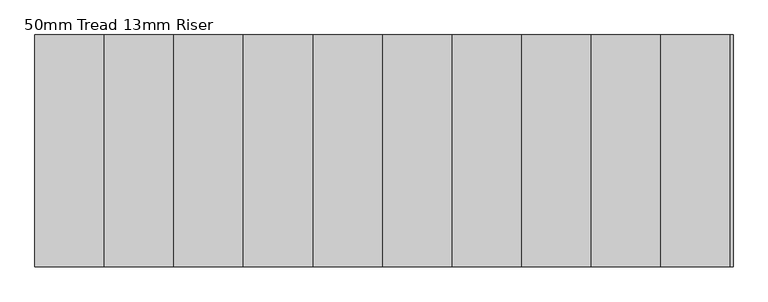
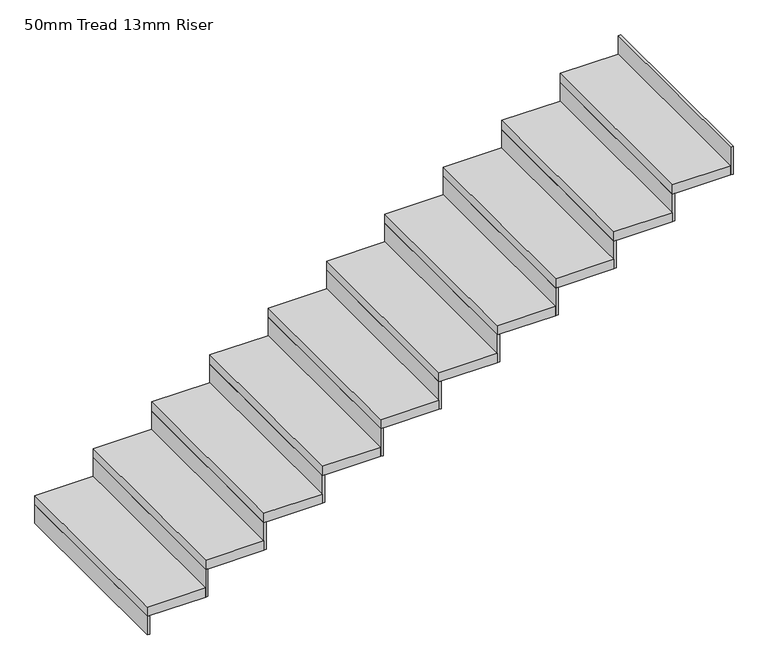
"""IFC4 building model written with IfcOpenShell, lengths in millimetres: stair flight geometry, 50mm Tread 13mm Riser."""

from ifc_helpers import new_model, si_unit, frame, origin, origin_with_axes, place, context, project, spatial, polyline, outline, extrude, source, transform, mapped, element, save


def stair_flight_50mm_tread_13mm_riser_b7d47cc6(model_context):
    return source(origin(), model_context, "Body", "SweptSolid", [
        extrude(outline(polyline([(1701.3435815, -3974.091395), (1688.8435815, -3974.091395), (1688.8435815, -2974.091395), (1701.3435815, -2974.091395), (1701.3435815, -3974.091395)])), origin_with_axes(), (0.0, 0.0, 1.0), 100.0),
        extrude(outline(polyline([(1988.8435815, -2974.091395), (1988.8435815, -3974.091395), (1688.8435815, -3974.091395), (1688.8435815, -2974.091395), (1988.8435815, -2974.091395)])), frame((0.0, 0.0, 100.0), z_axis=(0.0, 0.0, 1.0), x_axis=(1.0, 0.0, 0.0)), (0.0, 0.0, 1.0), 50.0),
        extrude(outline(polyline([(2001.3435815, -3974.091395), (1988.8435815, -3974.091395), (1988.8435815, -2974.091395), (2001.3435815, -2974.091395), (2001.3435815, -3974.091395)])), frame((0.0, 0.0, 100.0), z_axis=(0.0, 0.0, 1.0), x_axis=(1.0, 0.0, 0.0)), (0.0, 0.0, 1.0), 150.0),
        extrude(outline(polyline([(2288.8435815, -2974.091395), (2288.8435815, -3974.091395), (1988.8435815, -3974.091395), (1988.8435815, -2974.091395), (2288.8435815, -2974.091395)])), frame((0.0, 0.0, 250.0), z_axis=(0.0, 0.0, 1.0), x_axis=(1.0, 0.0, 0.0)), (0.0, 0.0, 1.0), 50.0),
        extrude(outline(polyline([(2301.3435815, -3974.091395), (2288.8435815, -3974.091395), (2288.8435815, -2974.091395), (2301.3435815, -2974.091395), (2301.3435815, -3974.091395)])), frame((0.0, 0.0, 250.0), z_axis=(0.0, 0.0, 1.0), x_axis=(1.0, 0.0, 0.0)), (0.0, 0.0, 1.0), 150.0),
        extrude(outline(polyline([(2588.8435815, -2974.091395), (2588.8435815, -3974.091395), (2288.8435815, -3974.091395), (2288.8435815, -2974.091395), (2588.8435815, -2974.091395)])), frame((0.0, 0.0, 400.0), z_axis=(0.0, 0.0, 1.0), x_axis=(1.0, 0.0, 0.0)), (0.0, 0.0, 1.0), 50.0),
        extrude(outline(polyline([(2601.3435815, -3974.091395), (2588.8435815, -3974.091395), (2588.8435815, -2974.091395), (2601.3435815, -2974.091395), (2601.3435815, -3974.091395)])), frame((0.0, 0.0, 400.0), z_axis=(0.0, 0.0, 1.0), x_axis=(1.0, 0.0, 0.0)), (0.0, 0.0, 1.0), 150.0),
        extrude(outline(polyline([(2888.8435815, -2974.091395), (2888.8435815, -3974.091395), (2588.8435815, -3974.091395), (2588.8435815, -2974.091395), (2888.8435815, -2974.091395)])), frame((0.0, 0.0, 550.0), z_axis=(0.0, 0.0, 1.0), x_axis=(1.0, 0.0, 0.0)), (0.0, 0.0, 1.0), 50.0),
        extrude(outline(polyline([(2901.3435815, -3974.091395), (2888.8435815, -3974.091395), (2888.8435815, -2974.091395), (2901.3435815, -2974.091395), (2901.3435815, -3974.091395)])), frame((0.0, 0.0, 550.0), z_axis=(0.0, 0.0, 1.0), x_axis=(1.0, 0.0, 0.0)), (0.0, 0.0, 1.0), 150.0),
        extrude(outline(polyline([(3188.8435815, -2974.091395), (3188.8435815, -3974.091395), (2888.8435815, -3974.091395), (2888.8435815, -2974.091395), (3188.8435815, -2974.091395)])), frame((0.0, 0.0, 700.0), z_axis=(0.0, 0.0, 1.0), x_axis=(1.0, 0.0, 0.0)), (0.0, 0.0, 1.0), 50.0),
        extrude(outline(polyline([(3201.3435815, -3974.091395), (3188.8435815, -3974.091395), (3188.8435815, -2974.091395), (3201.3435815, -2974.091395), (3201.3435815, -3974.091395)])), frame((0.0, 0.0, 700.0), z_axis=(0.0, 0.0, 1.0), x_axis=(1.0, 0.0, 0.0)), (0.0, 0.0, 1.0), 150.0),
        extrude(outline(polyline([(3488.8435815, -2974.091395), (3488.8435815, -3974.091395), (3188.8435815, -3974.091395), (3188.8435815, -2974.091395), (3488.8435815, -2974.091395)])), frame((0.0, 0.0, 850.0), z_axis=(0.0, 0.0, 1.0), x_axis=(1.0, 0.0, 0.0)), (0.0, 0.0, 1.0), 50.0),
        extrude(outline(polyline([(3501.3435815, -3974.091395), (3488.8435815, -3974.091395), (3488.8435815, -2974.091395), (3501.3435815, -2974.091395), (3501.3435815, -3974.091395)])), frame((0.0, 0.0, 850.0), z_axis=(0.0, 0.0, 1.0), x_axis=(1.0, 0.0, 0.0)), (0.0, 0.0, 1.0), 150.0),
        extrude(outline(polyline([(3788.8435815, -2974.091395), (3788.8435815, -3974.091395), (3488.8435815, -3974.091395), (3488.8435815, -2974.091395), (3788.8435815, -2974.091395)])), frame((0.0, 0.0, 1000.0), z_axis=(0.0, 0.0, 1.0), x_axis=(1.0, 0.0, 0.0)), (0.0, 0.0, 1.0), 50.0),
        extrude(outline(polyline([(3801.3435815, -3974.091395), (3788.8435815, -3974.091395), (3788.8435815, -2974.091395), (3801.3435815, -2974.091395), (3801.3435815, -3974.091395)])), frame((0.0, 0.0, 1000.0), z_axis=(0.0, 0.0, 1.0), x_axis=(1.0, 0.0, 0.0)), (0.0, 0.0, 1.0), 150.0),
        extrude(outline(polyline([(4088.8435815, -2974.091395), (4088.8435815, -3974.091395), (3788.8435815, -3974.091395), (3788.8435815, -2974.091395), (4088.8435815, -2974.091395)])), frame((0.0, 0.0, 1150.0), z_axis=(0.0, 0.0, 1.0), x_axis=(1.0, 0.0, 0.0)), (0.0, 0.0, 1.0), 50.0),
        extrude(outline(polyline([(4101.3435815, -3974.091395), (4088.8435815, -3974.091395), (4088.8435815, -2974.091395), (4101.3435815, -2974.091395), (4101.3435815, -3974.091395)])), frame((0.0, 0.0, 1150.0), z_axis=(0.0, 0.0, 1.0), x_axis=(1.0, 0.0, 0.0)), (0.0, 0.0, 1.0), 150.0),
        extrude(outline(polyline([(4388.8435815, -2974.091395), (4388.8435815, -3974.091395), (4088.8435815, -3974.091395), (4088.8435815, -2974.091395), (4388.8435815, -2974.091395)])), frame((0.0, 0.0, 1300.0), z_axis=(0.0, 0.0, 1.0), x_axis=(1.0, 0.0, 0.0)), (0.0, 0.0, 1.0), 50.0),
        extrude(outline(polyline([(4401.3435815, -3974.091395), (4388.8435815, -3974.091395), (4388.8435815, -2974.091395), (4401.3435815, -2974.091395), (4401.3435815, -3974.091395)])), frame((0.0, 0.0, 1300.0), z_axis=(0.0, 0.0, 1.0), x_axis=(1.0, 0.0, 0.0)), (0.0, 0.0, 1.0), 150.0),
        extrude(outline(polyline([(4701.3435815, -3974.091395), (4688.8435815, -3974.091395), (4688.8435815, -2974.091395), (4701.3435815, -2974.091395), (4701.3435815, -3974.091395)])), frame((0.0, 0.0, 1450.0), z_axis=(0.0, 0.0, 1.0), x_axis=(1.0, 0.0, 0.0)), (0.0, 0.0, 1.0), 150.0),
        extrude(outline(polyline([(4688.8435815, -2974.091395), (4688.8435815, -3974.091395), (4388.8435815, -3974.091395), (4388.8435815, -2974.091395), (4688.8435815, -2974.091395)])), frame((0.0, 0.0, 1450.0), z_axis=(0.0, 0.0, 1.0), x_axis=(1.0, 0.0, 0.0)), (0.0, 0.0, 1.0), 50.0),
    ])


if __name__ == "__main__":
    model = new_model("IFC4")
    model_context = context("Model", 3, world=origin())
    ifc_project = project(units=[si_unit("LENGTHUNIT", "METRE", prefix="MILLI")], contexts=[model_context])
    site = spatial("IfcSite", under=ifc_project)
    building = spatial("IfcBuilding", under=site)
    placement = place(None, origin())
    stair_flight_50mm_tread_13mm_riser_shape = stair_flight_50mm_tread_13mm_riser_b7d47cc6(model_context)
    element("IfcStairFlight", 1, ObjectType="50mm Tread 13mm Riser", at=placement, inside=building, context=model_context, shape_type="MappedRepresentation", body=[
        mapped(stair_flight_50mm_tread_13mm_riser_shape, transform((0.0, 0.0, 0.0), x_axis=(1.0, 0.0, 0.0), y_axis=(0.0, 1.0, 0.0), z_axis=(0.0, 0.0, 1.0))),
    ])
    save(model, "model.ifc")
